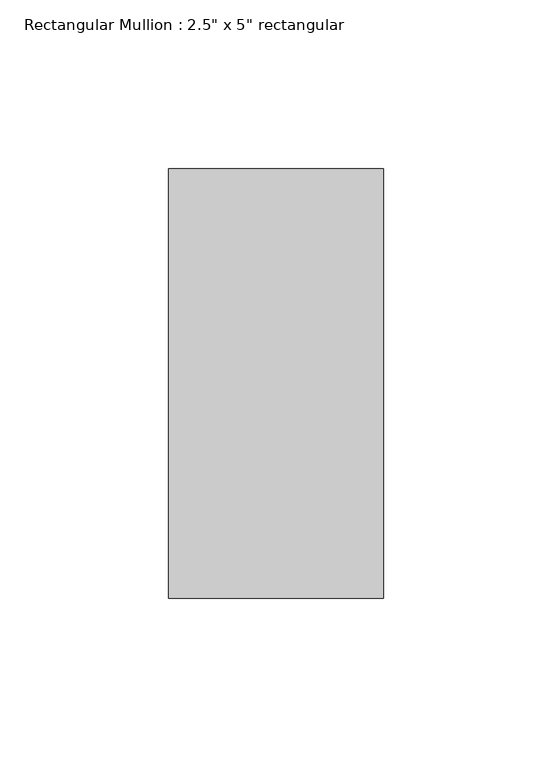
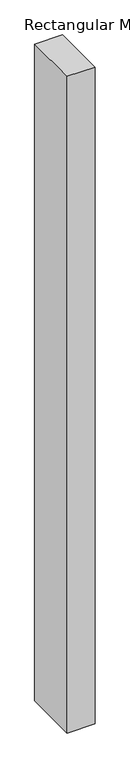
"""IFC4 building model written with IfcOpenShell, lengths in millimetres: member geometry."""

from ifc_helpers import new_model, si_unit, frame, origin, place, context, project, spatial, polyline, outline, extrude, source, transform, mapped, element, save


def member_3d617b91(model_context):
    return source(origin(), model_context, "Body", "SweptSolid", [
        extrude(outline(polyline([(0.0, 63.5), (0.0, -63.5), (-63.5, -63.5), (-63.5, 63.5), (0.0, 63.5)])), frame((0.0, 0.0, -1569.5186051), z_axis=(0.0, 0.0, 1.0), x_axis=(1.0, 0.0, 0.0)), (0.0, 0.0, 1.0), 1569.5186051),
    ])


if __name__ == "__main__":
    model = new_model("IFC4")
    model_context = context("Model", 3, world=origin())
    ifc_project = project(units=[si_unit("LENGTHUNIT", "METRE", prefix="MILLI")], contexts=[model_context])
    site = spatial("IfcSite", under=ifc_project)
    building = spatial("IfcBuilding", under=site)
    placement = place(None, origin())
    member_shape = member_3d617b91(model_context)
    element("IfcMember", 1, ObjectType="Rectangular Mullion : 2.5\" x 5\" rectangular", at=placement, inside=building, context=model_context, shape_type="MappedRepresentation", body=[
        mapped(member_shape, transform((0.0, 0.0, 0.0), x_axis=(1.0, 0.0, 0.0), y_axis=(0.0, 1.0, 0.0), z_axis=(0.0, 0.0, 1.0))),
    ])
    save(model, "model.ifc")

# Revit data of these elements
# Type "Rectangular Mullion : 2.5\" x 5\" rectangular"
#   built-in parameter 1007304 = 0.416667 (stored number, unit not read)
#   built-in parameter 1007301 = 0.104167 (stored number, unit not read)
#   built-in parameter 1007300 = 0.104167 (stored number, unit not read)
# Element 1 (IfcMember, "Rectangular Mullion : 2.5\" x 5\" rectangular")
#   Materials on its faces: "Aluminum"
# Materials
#   "Aluminum": class "Metal", colour RGB 247 247 247, transparency 0, Description = "Aluminum 6061", Cost = 0
